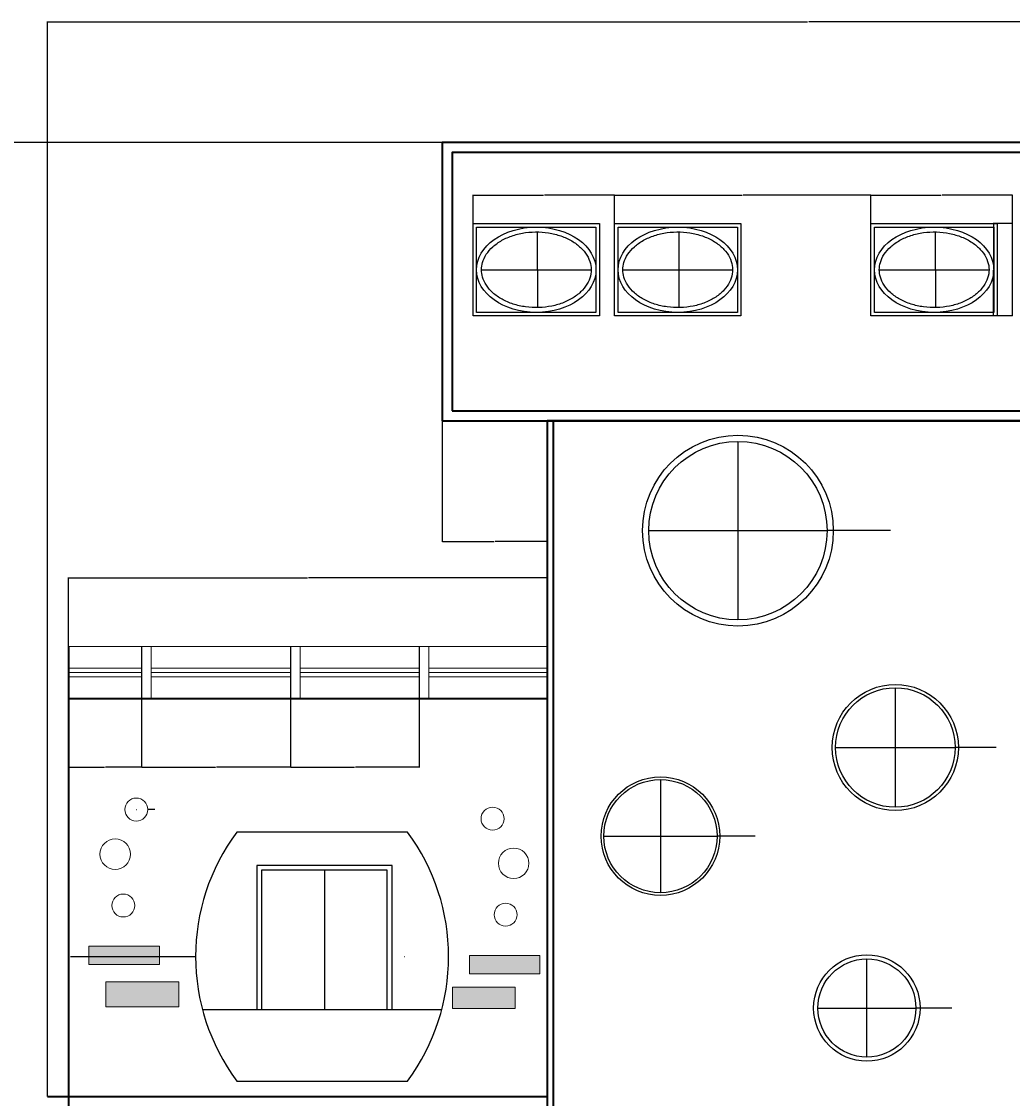
# Model space of a CAD drawing. Units: inches. Extents: x 328 to 2318, y 647 to 2548.
# Tile 4 of 5: x 1040 to 1799, y 1724 to 2548. Entities that reach past the tile are written whole.
import ezdxf

# ---------------------------------------------------------------- set-up
doc = ezdxf.new("R2010")
doc.units = ezdxf.units.IN
doc.header["$MEASUREMENT"] = 0
for name, color, linetype, lineweight in [('A-ANNO-DIMS', 2, 'Continuous', 18), ('A-ELEV', 7, 'Continuous', 35), ('A-ELEV-ORNM', 7, 'Continuous', 18), ('A-GLAZ', 4, 'Continuous', 25), ('A-ROOF', 7, 'Continuous', 35), ('A-ROOF-HRAL', 8, 'Continuous', 18)]:
    doc.layers.add(name, color=color, linetype=linetype, lineweight=lineweight)
doc.layers.add('A-ELEV-ORNM-PATT', color=18, linetype='Continuous', lineweight=13, true_color=0x000000)
doc.styles.get("Standard").update_dxf_attribs({"font": 'arial.ttf'})
doc.dimstyles.get("Standard").update_dxf_attribs({"dimtxt": 0.18, "dimasz": 0.18, "dimexe": 0.18, "dimexo": 0.0625, "dimgap": 0.09, "dimtad": 0, "dimtih": 1, "dimtoh": 1, "dimdec": 4, "dimzin": 0, "dimdsep": 46, "dimtxsty": 'Standard', "dimcen": 0.09, "dimadec": 0, "dimazin": 0, "dimtfac": 1, "dimtdec": 4, "dimtofl": 0, "dimtmove": 0, "dimatfit": 3, "dimfxl": 1, "dimtolj": 1, "dimtzin": 0, "dimarcsym": 0})

# ---------------------------------------------------------------- blocks, each defined once
blk = doc.blocks.new('WIN-ELEV-CURVED-SURROUND')
for p, q in [((162.11, 190.69), (31.57, 190.69)), ((98.64, 161.37), (98.64, 54.8)), ((5.23, 54.8), (188.45, 54.8)), ((31.57, 0), (162.11, 0))]:
    blk.add_line(p, q)
for points in [[(150.48, 54.8), (150.48, 165.07), (46.8, 165.07), (46.8, 54.8)], [(146.78, 54.8), (146.78, 161.37), (50.49, 161.37), (50.49, 54.8)]]:
    blk.add_lwpolyline(points)
for centre, start, end in [((159.76, 95.35), 143.35881, 216.64119), ((33.92, 95.35), 323.35881, 36.64119)]:
    blk.add_arc(centre, 159.76, start, end)
blk = doc.blocks.new('WIN-ELEV-OVAL')
for p, q in [((49.54, 6.37), (49.37, 64.33)), ((6.36, 35.36), (90.36, 35.36))]:
    blk.add_line(p, q)
for points in [[(0, 70.7), (96.72, 70.7), (96.72, 0), (0, 0)], [(2.67, 68.03), (94.06, 68.03), (94.06, 2.67), (2.67, 2.67)]]:
    blk.add_lwpolyline(points, close=True)
blk.add_ellipse((48.36, 35.35), major_axis=(-45.7, 0), ratio=0.715242)
blk.add_open_spline([(6.36, 35.35), (6.36, 33.47), (6.63, 31.58), (7.79, 27.59), (8.77, 25.48), (11.44, 21.43), (13.14, 19.48), (17.17, 15.88), (19.51, 14.22), (24.72, 11.33), (27.59, 10.09), (33.68, 8.11), (36.9, 7.38), (43.51, 6.46), (46.9, 6.28), (53.63, 6.5), (56.98, 6.89), (63.44, 8.21), (66.55, 9.15), (72.35, 11.49), (75.04, 12.9), (79.83, 16.09), (81.94, 17.87), (85.48, 21.67), (86.9, 23.7), (89.04, 27.86), (89.75, 29.99), (90.45, 34.29), (90.45, 36.45), (89.74, 40.75), (89.02, 42.88), (86.88, 47.04), (85.45, 49.06), (81.9, 52.86), (79.79, 54.64), (74.99, 57.83), (72.3, 59.23), (66.49, 61.57), (63.38, 62.5), (56.92, 63.82), (53.57, 64.21), (46.83, 64.41), (43.45, 64.23), (36.84, 63.31), (33.62, 62.57), (27.53, 60.59), (24.67, 59.35), (19.47, 56.45), (17.13, 54.79), (13.1, 51.18), (11.41, 49.23), (8.75, 45.18), (7.78, 43.07), (6.63, 39.09), (6.36, 37.22), (6.36, 35.35)], degree=3, knots=[0, 0, 0, 0, 0.205219, 0.205219, 0.440189, 0.440189, 0.675159, 0.675159, 0.910128, 0.910128, 1.145098, 1.145098, 1.380068, 1.380068, 1.615038, 1.615038, 1.850008, 1.850008, 2.084978, 2.084978, 2.319948, 2.319948, 2.554918, 2.554918, 2.789887, 2.789887, 3.024857, 3.024857, 3.259827, 3.259827, 3.494797, 3.494797, 3.729767, 3.729767, 3.964737, 3.964737, 4.199707, 4.199707, 4.434676, 4.434676, 4.669646, 4.669646, 4.904616, 4.904616, 5.139586, 5.139586, 5.374556, 5.374556, 5.609526, 5.609526, 5.844496, 5.844496, 6.079466, 6.079466, 6.283185, 6.283185, 6.283185, 6.283185])
blk = doc.blocks.new('FACADE-THREE-ROUNDELS')
for centre, radius in [((27.83, 82.27), 8.8), ((11.7, 48.09), 11.7), ((17.88, 8.77), 8.77)]:
    blk.add_circle(centre, radius)
blk = doc.blocks.new('POST-PARAPET')
blk.add_lwpolyline([(0, 0), (7.34, 0), (7.34, 39.76), (0, 39.76)], close=True)
blk = doc.blocks.new('*D8')
at = {"layer": 'A-ANNO-DIMS', "color": 0, "lineweight": -2, "transparency": 16777216}
for p, q in [((1798.98, 2393.44), (1784.36, 2393.44)), ((1784.54, 2393.26), (1784.54, 2358.27)), ((1784.54, 2322.92), (1784.54, 2357.91)), ((1798.98, 2322.74), (1784.36, 2322.74))]:
    blk.add_line(p, q, dxfattribs=at)
at = {"layer": 'A-ANNO-DIMS', "color": 0, "transparency": 16777216}
for points in [[(1784.51, 2393.26), (1784.57, 2393.26), (1784.54, 2393.44)], [(1784.51, 2322.92), (1784.57, 2322.92), (1784.54, 2322.74)]]:
    blk.add_solid(points, dxfattribs=at)
at = {"layer": 'Defpoints', "color": 0, "transparency": 16777216}
for p in [(1784.54, 2393.44), (1799.05, 2393.44), (1799.05, 2322.74)]:
    blk.add_point(p, dxfattribs=at)
at = {"layer": 'A-ANNO-DIMS', "color": 0, "transparency": 16777216, "insert": (1784.54, 2358.09), "char_height": 0.18, "attachment_point": 5}
blk.add_mtext('\\A1;71 TYP.', dxfattribs=at)
blk = doc.blocks.new('*D39')
at = {"layer": 'A-ANNO-DIMS', "color": 0, "lineweight": -2, "transparency": 16777216}
for p, q in [((1060.28, 1725.1), (1060.28, 2548.17)), ((2224.98, 2069.65), (2224.98, 2548.17)), ((1060.46, 2547.99), (1642.17, 2547.99)), ((2224.8, 2547.99), (1643.08, 2547.99))]:
    blk.add_line(p, q, dxfattribs=at)
at = {"layer": 'A-ANNO-DIMS', "color": 0, "transparency": 16777216}
for points in [[(1060.46, 2548.02), (1060.46, 2547.96), (1060.28, 2547.99)], [(2224.8, 2548.02), (2224.8, 2547.96), (2224.98, 2547.99)]]:
    blk.add_solid(points, dxfattribs=at)
at = {"layer": 'Defpoints', "color": 0, "transparency": 16777216}
for p in [(2224.98, 2547.99), (2224.98, 2069.59), (1060.28, 1725.04)]:
    blk.add_point(p, dxfattribs=at)
at = {"layer": 'A-ANNO-DIMS', "color": 0, "transparency": 16777216, "insert": (1642.63, 2547.99), "char_height": 0.18, "attachment_point": 5}
blk.add_mtext('\\A1;1164.7', dxfattribs=at)
blk = doc.blocks.new('*D40')
at = {"layer": 'A-ANNO-DIMS', "color": 0, "lineweight": -2, "transparency": 16777216}
for p, q in [((1362.32, 2455.54), (967.65, 2455.54)), ((967.83, 2455.36), (967.83, 1622.35)), ((967.83, 788.97), (967.83, 1621.98)), ((1076.36, 788.79), (967.65, 788.79))]:
    blk.add_line(p, q, dxfattribs=at)
at = {"layer": 'A-ANNO-DIMS', "color": 0, "transparency": 16777216}
for points in [[(967.8, 2455.36), (967.86, 2455.36), (967.83, 2455.54)], [(967.8, 788.97), (967.86, 788.97), (967.83, 788.79)]]:
    blk.add_solid(points, dxfattribs=at)
at = {"layer": 'Defpoints', "color": 0, "transparency": 16777216}
for p in [(967.83, 2455.54), (1362.39, 2455.54), (1076.43, 788.79)]:
    blk.add_point(p, dxfattribs=at)
at = {"layer": 'A-ANNO-DIMS', "color": 0, "transparency": 16777216, "insert": (967.83, 1622.16), "char_height": 0.18, "attachment_point": 5}
blk.add_mtext('\\A1;1666.7', dxfattribs=at)
blk = doc.blocks.new('*D41')
at = {"layer": 'A-ANNO-DIMS', "color": 0, "lineweight": -2, "transparency": 16777216}
for p, q in [((1076.43, 2029.9), (1076.43, 2122.46)), ((1076.61, 2122.28), (1259.22, 2122.28)), ((1442.63, 2122.28), (1260.01, 2122.28)), ((1442.81, 2029.9), (1442.81, 2122.46))]:
    blk.add_line(p, q, dxfattribs=at)
at = {"layer": 'A-ANNO-DIMS', "color": 0, "transparency": 16777216}
for points in [[(1076.61, 2122.31), (1076.61, 2122.25), (1076.43, 2122.28)], [(1442.63, 2122.31), (1442.63, 2122.25), (1442.81, 2122.28)]]:
    blk.add_solid(points, dxfattribs=at)
at = {"layer": 'Defpoints', "color": 0, "transparency": 16777216}
for p in [(1442.81, 2122.28), (1076.43, 2029.83), (1442.81, 2029.83)]:
    blk.add_point(p, dxfattribs=at)
at = {"layer": 'A-ANNO-DIMS', "color": 0, "transparency": 16777216, "insert": (1259.62, 2122.28), "char_height": 0.18, "attachment_point": 5}
blk.add_mtext('\\A1;366.4', dxfattribs=at)
blk = doc.blocks.new('*D47')
at = {"layer": 'A-ANNO-DIMS', "color": 0, "lineweight": -2, "transparency": 16777216}
for p, q in [((1362.39, 2242.37), (1362.39, 2149.8)), ((1442.81, 2242.37), (1442.81, 2149.8)), ((1362.57, 2149.98), (1402.2, 2149.98)), ((1442.63, 2149.98), (1402.99, 2149.98))]:
    blk.add_line(p, q, dxfattribs=at)
at = {"layer": 'A-ANNO-DIMS', "color": 0, "transparency": 16777216}
for points in [[(1362.57, 2150.01), (1362.57, 2149.95), (1362.39, 2149.98)], [(1442.63, 2150.01), (1442.63, 2149.95), (1442.81, 2149.98)]]:
    blk.add_solid(points, dxfattribs=at)
at = {"layer": 'Defpoints', "color": 0, "transparency": 16777216}
for p in [(1362.39, 2242.43), (1442.81, 2242.43), (1362.39, 2149.98)]:
    blk.add_point(p, dxfattribs=at)
at = {"layer": 'A-ANNO-DIMS', "color": 0, "transparency": 16777216, "insert": (1402.6, 2149.98), "char_height": 0.18, "attachment_point": 5}
blk.add_mtext('\\A1;80.42', dxfattribs=at)
blk = doc.blocks.new('*D50')
at = {"layer": 'A-ANNO-DIMS', "color": 0, "lineweight": -2, "transparency": 16777216}
for p, q in [((1386.14, 2322.8), (1386.14, 2415.37)), ((1386.32, 2415.19), (1439.9, 2415.19)), ((1494.26, 2415.19), (1440.67, 2415.19)), ((1494.44, 2322.8), (1494.44, 2415.37))]:
    blk.add_line(p, q, dxfattribs=at)
at = {"layer": 'A-ANNO-DIMS', "color": 0, "transparency": 16777216}
for points in [[(1386.32, 2415.22), (1386.32, 2415.16), (1386.14, 2415.19)], [(1494.26, 2415.22), (1494.26, 2415.16), (1494.44, 2415.19)]]:
    blk.add_solid(points, dxfattribs=at)
at = {"layer": 'Defpoints', "color": 0, "transparency": 16777216}
for p in [(1494.44, 2415.19), (1386.14, 2322.74), (1494.44, 2322.74)]:
    blk.add_point(p, dxfattribs=at)
at = {"layer": 'A-ANNO-DIMS', "color": 0, "transparency": 16777216, "insert": (1440.29, 2415.19), "char_height": 0.18, "attachment_point": 5}
blk.add_mtext('\\A1;108.3', dxfattribs=at)
blk = doc.blocks.new('*D51')
at = {"layer": 'A-ANNO-DIMS', "color": 0, "lineweight": -2, "transparency": 16777216}
for p, q in [((1494.44, 2322.8), (1494.44, 2415.37)), ((1494.62, 2415.19), (1592.21, 2415.19)), ((1690.56, 2415.19), (1592.98, 2415.19)), ((1690.74, 2322.8), (1690.74, 2415.37))]:
    blk.add_line(p, q, dxfattribs=at)
at = {"layer": 'A-ANNO-DIMS', "color": 0, "transparency": 16777216}
for points in [[(1494.62, 2415.22), (1494.62, 2415.16), (1494.44, 2415.19)], [(1690.56, 2415.22), (1690.56, 2415.16), (1690.74, 2415.19)]]:
    blk.add_solid(points, dxfattribs=at)
at = {"layer": 'Defpoints', "color": 0, "transparency": 16777216}
for p in [(1690.74, 2415.19), (1494.44, 2322.74), (1690.74, 2322.74)]:
    blk.add_point(p, dxfattribs=at)
at = {"layer": 'A-ANNO-DIMS', "color": 0, "transparency": 16777216, "insert": (1592.59, 2415.19), "char_height": 0.18, "attachment_point": 5}
blk.add_mtext('\\A1;196.3', dxfattribs=at)
blk = doc.blocks.new('*D52')
at = {"layer": 'A-ANNO-DIMS', "color": 0, "lineweight": -2, "transparency": 16777216}
for p, q in [((1690.74, 2322.8), (1690.74, 2415.37)), ((1690.92, 2415.19), (1744.51, 2415.19)), ((1798.87, 2415.19), (1745.28, 2415.19)), ((1799.05, 2322.8), (1799.05, 2415.37))]:
    blk.add_line(p, q, dxfattribs=at)
at = {"layer": 'A-ANNO-DIMS', "color": 0, "transparency": 16777216}
for points in [[(1690.92, 2415.22), (1690.92, 2415.16), (1690.74, 2415.19)], [(1798.87, 2415.22), (1798.87, 2415.16), (1799.05, 2415.19)]]:
    blk.add_solid(points, dxfattribs=at)
at = {"layer": 'Defpoints', "color": 0, "transparency": 16777216}
for p in [(1799.05, 2415.19), (1690.74, 2322.74), (1799.05, 2322.74)]:
    blk.add_point(p, dxfattribs=at)
at = {"layer": 'A-ANNO-DIMS', "color": 0, "transparency": 16777216, "insert": (1744.89, 2415.19), "char_height": 0.18, "attachment_point": 5}
blk.add_mtext('\\A1;108.3', dxfattribs=at)
blk = doc.blocks.new('*D62')
at = {"layer": 'A-ANNO-DIMS', "color": 0, "lineweight": -2, "transparency": 16777216}
for p, q in [((1076.43, 2069.53), (1076.43, 1976.96)), ((1132.18, 2069.53), (1132.18, 1976.96)), ((1076.61, 1977.14), (1103.91, 1977.14)), ((1132, 1977.14), (1104.7, 1977.14))]:
    blk.add_line(p, q, dxfattribs=at)
at = {"layer": 'A-ANNO-DIMS', "color": 0, "transparency": 16777216}
for points in [[(1076.61, 1977.17), (1076.61, 1977.11), (1076.43, 1977.14)], [(1132, 1977.17), (1132, 1977.11), (1132.18, 1977.14)]]:
    blk.add_solid(points, dxfattribs=at)
at = {"layer": 'Defpoints', "color": 0, "transparency": 16777216}
for p in [(1076.43, 2069.59), (1132.18, 2069.59), (1076.43, 1977.14)]:
    blk.add_point(p, dxfattribs=at)
at = {"layer": 'A-ANNO-DIMS', "color": 0, "transparency": 16777216, "insert": (1104.3, 1977.14), "char_height": 0.18, "attachment_point": 5}
blk.add_mtext('\\A1;55.76', dxfattribs=at)
blk = doc.blocks.new('*D63')
at = {"layer": 'A-ANNO-DIMS', "color": 0, "lineweight": -2, "transparency": 16777216}
for p, q in [((1132.18, 2069.53), (1132.18, 1976.96)), ((1246.42, 2069.53), (1246.42, 1976.96)), ((1132.36, 1977.14), (1188.85, 1977.14)), ((1246.24, 1977.14), (1189.76, 1977.14))]:
    blk.add_line(p, q, dxfattribs=at)
at = {"layer": 'A-ANNO-DIMS', "color": 0, "transparency": 16777216}
for points in [[(1132.36, 1977.17), (1132.36, 1977.11), (1132.18, 1977.14)], [(1246.24, 1977.17), (1246.24, 1977.11), (1246.42, 1977.14)]]:
    blk.add_solid(points, dxfattribs=at)
at = {"layer": 'Defpoints', "color": 0, "transparency": 16777216}
for p in [(1132.18, 2069.59), (1246.42, 2069.59), (1132.18, 1977.14)]:
    blk.add_point(p, dxfattribs=at)
at = {"layer": 'A-ANNO-DIMS', "color": 0, "transparency": 16777216, "insert": (1189.3, 1977.14), "char_height": 0.18, "attachment_point": 5}
blk.add_mtext('\\A1;114.24', dxfattribs=at)
blk = doc.blocks.new('*D64')
at = {"layer": 'A-ANNO-DIMS', "color": 0, "lineweight": -2, "transparency": 16777216}
for p, q in [((1246.42, 2069.53), (1246.42, 1976.96)), ((1344.93, 2069.53), (1344.93, 1976.96)), ((1246.6, 1977.14), (1295.28, 1977.14)), ((1344.75, 1977.14), (1296.07, 1977.14))]:
    blk.add_line(p, q, dxfattribs=at)
at = {"layer": 'A-ANNO-DIMS', "color": 0, "transparency": 16777216}
for points in [[(1246.6, 1977.17), (1246.6, 1977.11), (1246.42, 1977.14)], [(1344.75, 1977.17), (1344.75, 1977.11), (1344.93, 1977.14)]]:
    blk.add_solid(points, dxfattribs=at)
at = {"layer": 'Defpoints', "color": 0, "transparency": 16777216}
for p in [(1246.42, 2069.59), (1344.93, 2069.59), (1246.42, 1977.14)]:
    blk.add_point(p, dxfattribs=at)
at = {"layer": 'A-ANNO-DIMS', "color": 0, "transparency": 16777216, "insert": (1295.68, 1977.14), "char_height": 0.18, "attachment_point": 5}
blk.add_mtext('\\A1;98.52', dxfattribs=at)
blk = doc.blocks.new('*D68')
at = {"layer": 'A-ANNO-DIMS', "color": 0, "lineweight": -2, "transparency": 16777216}
for p, q in [((1077.79, 1832.22), (1173.47, 1832.22)), ((1333.32, 1832.22), (1333.5, 1832.22)), ((1333.41, 1832.13), (1333.41, 1832.31))]:
    blk.add_line(p, q, dxfattribs=at)
at = {"layer": 'A-ANNO-DIMS', "color": 0, "transparency": 16777216}
blk.add_solid([(1173.47, 1832.25), (1173.47, 1832.19), (1173.65, 1832.22)], dxfattribs=at)
at = {"layer": 'Defpoints', "color": 0, "transparency": 16777216}
for p in [(1173.65, 1832.22), (1333.41, 1832.22)]:
    blk.add_point(p, dxfattribs=at)
at = {"layer": 'A-ANNO-DIMS', "color": 0, "transparency": 16777216, "insert": (1076.99, 1832.22), "char_height": 0.18, "attachment_point": 5}
blk.add_mtext('\\A1;16X R159.76', dxfattribs=at)
blk = doc.blocks.new('*D70')
at = {"layer": 'A-ANNO-DIMS', "color": 0, "lineweight": -2, "transparency": 16777216}
for p, q in [((1128.14, 1944.79), (1128.32, 1944.79)), ((1128.23, 1944.7), (1128.23, 1944.88)), ((1142.31, 1944.79), (1137.21, 1944.79))]:
    blk.add_line(p, q, dxfattribs=at)
at = {"layer": 'A-ANNO-DIMS', "color": 0, "transparency": 16777216}
blk.add_solid([(1137.21, 1944.82), (1137.21, 1944.76), (1137.03, 1944.79)], dxfattribs=at)
at = {"layer": 'Defpoints', "color": 0, "transparency": 16777216}
for p in [(1119.43, 1944.79), (1137.03, 1944.79)]:
    blk.add_point(p, dxfattribs=at)
at = {"layer": 'A-ANNO-DIMS', "color": 0, "transparency": 16777216, "insert": (1143.12, 1944.79), "char_height": 0.18, "attachment_point": 5}
blk.add_mtext('\\A1;16X ∅17.595', dxfattribs=at)
blk = doc.blocks.new('*D72')
at = {"layer": 'A-ANNO-DIMS', "color": 0, "lineweight": -2, "transparency": 16777216}
for p, q in [((1588.76, 2158.33), (1588.94, 2158.33)), ((1588.85, 2158.24), (1588.85, 2158.42)), ((1705.7, 2158.33), (1662.06, 2158.33))]:
    blk.add_line(p, q, dxfattribs=at)
at = {"layer": 'A-ANNO-DIMS', "color": 0, "transparency": 16777216}
blk.add_solid([(1662.06, 2158.36), (1662.06, 2158.3), (1661.88, 2158.33)], dxfattribs=at)
at = {"layer": 'Defpoints', "color": 0, "transparency": 16777216}
for p in [(1515.83, 2158.33), (1661.88, 2158.33)]:
    blk.add_point(p, dxfattribs=at)
at = {"layer": 'A-ANNO-DIMS', "color": 0, "transparency": 16777216, "insert": (1706.26, 2158.33), "char_height": 0.18, "attachment_point": 5}
blk.add_mtext('\\A1;∅146.05', dxfattribs=at)
blk = doc.blocks.new('*D73')
at = {"layer": 'A-ANNO-DIMS', "color": 0, "lineweight": -2, "transparency": 16777216}
for p, q in [((1588.76, 2158.33), (1588.94, 2158.33)), ((1588.85, 2158.24), (1588.85, 2158.42)), ((1698.11, 2158.33), (1657.32, 2158.33))]:
    blk.add_line(p, q, dxfattribs=at)
at = {"layer": 'A-ANNO-DIMS', "color": 0, "transparency": 16777216}
blk.add_solid([(1657.32, 2158.36), (1657.32, 2158.3), (1657.14, 2158.33)], dxfattribs=at)
at = {"layer": 'Defpoints', "color": 0, "transparency": 16777216}
for p in [(1520.57, 2158.33), (1657.14, 2158.33)]:
    blk.add_point(p, dxfattribs=at)
at = {"layer": 'A-ANNO-DIMS', "color": 0, "transparency": 16777216, "insert": (1698.67, 2158.33), "char_height": 0.18, "attachment_point": 5}
blk.add_mtext('\\A1;∅136.57', dxfattribs=at)
blk = doc.blocks.new('*D78')
at = {"layer": 'A-ANNO-DIMS', "color": 0, "lineweight": -2, "transparency": 16777216}
for p, q in [((1709.27, 1992.31), (1709.45, 1992.31)), ((1709.36, 1992.22), (1709.36, 1992.4)), ((1786.65, 1992.31), (1757.84, 1992.31))]:
    blk.add_line(p, q, dxfattribs=at)
at = {"layer": 'A-ANNO-DIMS', "color": 0, "transparency": 16777216}
blk.add_solid([(1757.84, 1992.34), (1757.84, 1992.28), (1757.66, 1992.31)], dxfattribs=at)
at = {"layer": 'Defpoints', "color": 0, "transparency": 16777216}
for p in [(1661.05, 1992.31), (1757.66, 1992.31)]:
    blk.add_point(p, dxfattribs=at)
at = {"layer": 'A-ANNO-DIMS', "color": 0, "transparency": 16777216, "insert": (1787.12, 1992.31), "char_height": 0.18, "attachment_point": 5}
blk.add_mtext('\\A1;∅96.61', dxfattribs=at)
blk = doc.blocks.new('*D79')
at = {"layer": 'A-ANNO-DIMS', "color": 0, "lineweight": -2, "transparency": 16777216}
for p, q in [((1709.27, 1992.31), (1709.45, 1992.31)), ((1709.36, 1992.22), (1709.36, 1992.4)), ((1782.57, 1992.31), (1755.29, 1992.31))]:
    blk.add_line(p, q, dxfattribs=at)
at = {"layer": 'A-ANNO-DIMS', "color": 0, "transparency": 16777216}
blk.add_solid([(1755.29, 1992.34), (1755.29, 1992.28), (1755.11, 1992.31)], dxfattribs=at)
at = {"layer": 'Defpoints', "color": 0, "transparency": 16777216}
for p in [(1663.6, 1992.31), (1755.11, 1992.31)]:
    blk.add_point(p, dxfattribs=at)
at = {"layer": 'A-ANNO-DIMS', "color": 0, "transparency": 16777216, "insert": (1783.04, 1992.31), "char_height": 0.18, "attachment_point": 5}
blk.add_mtext('\\A1;∅91.51', dxfattribs=at)
blk = doc.blocks.new('*D80')
at = {"layer": 'A-ANNO-DIMS', "color": 0, "lineweight": -2, "transparency": 16777216}
for p, q in [((1529.44, 1924.41), (1529.62, 1924.41)), ((1529.53, 1924.32), (1529.53, 1924.5)), ((1602.18, 1924.41), (1575.12, 1924.41))]:
    blk.add_line(p, q, dxfattribs=at)
at = {"layer": 'A-ANNO-DIMS', "color": 0, "transparency": 16777216}
blk.add_solid([(1575.12, 1924.44), (1575.12, 1924.38), (1574.94, 1924.41)], dxfattribs=at)
at = {"layer": 'Defpoints', "color": 0, "transparency": 16777216}
for p in [(1484.13, 1924.41), (1574.94, 1924.41)]:
    blk.add_point(p, dxfattribs=at)
at = {"layer": 'A-ANNO-DIMS', "color": 0, "transparency": 16777216, "insert": (1602.6, 1924.41), "char_height": 0.18, "attachment_point": 5}
blk.add_mtext('\\A1;∅90.8', dxfattribs=at)
blk = doc.blocks.new('*D81')
at = {"layer": 'A-ANNO-DIMS', "color": 0, "lineweight": -2, "transparency": 16777216}
for p, q in [((1529.44, 1924.41), (1529.62, 1924.41)), ((1529.53, 1924.32), (1529.53, 1924.5)), ((1598.88, 1924.41), (1573.05, 1924.41))]:
    blk.add_line(p, q, dxfattribs=at)
at = {"layer": 'A-ANNO-DIMS', "color": 0, "transparency": 16777216}
blk.add_solid([(1573.05, 1924.44), (1573.05, 1924.38), (1572.87, 1924.41)], dxfattribs=at)
at = {"layer": 'Defpoints', "color": 0, "transparency": 16777216}
for p in [(1486.19, 1924.41), (1572.87, 1924.41)]:
    blk.add_point(p, dxfattribs=at)
at = {"layer": 'A-ANNO-DIMS', "color": 0, "transparency": 16777216, "insert": (1599.37, 1924.41), "char_height": 0.18, "attachment_point": 5}
blk.add_mtext('\\A1;∅86.68', dxfattribs=at)
blk = doc.blocks.new('*D82')
at = {"layer": 'A-ANNO-DIMS', "color": 0, "lineweight": -2, "transparency": 16777216}
for p, q in [((1687.48, 1792.81), (1687.66, 1792.81)), ((1687.57, 1792.72), (1687.57, 1792.9)), ((1752.75, 1792.81), (1728.49, 1792.81))]:
    blk.add_line(p, q, dxfattribs=at)
at = {"layer": 'A-ANNO-DIMS', "color": 0, "transparency": 16777216}
blk.add_solid([(1728.49, 1792.84), (1728.49, 1792.78), (1728.31, 1792.81)], dxfattribs=at)
at = {"layer": 'Defpoints', "color": 0, "transparency": 16777216}
for p in [(1646.84, 1792.81), (1728.31, 1792.81)]:
    blk.add_point(p, dxfattribs=at)
at = {"layer": 'A-ANNO-DIMS', "color": 0, "transparency": 16777216, "insert": (1753.25, 1792.81), "char_height": 0.18, "attachment_point": 5}
blk.add_mtext('\\A1;∅81.48', dxfattribs=at)
blk = doc.blocks.new('*D83')
at = {"layer": 'A-ANNO-DIMS', "color": 0, "lineweight": -2, "transparency": 16777216}
for p, q in [((1687.48, 1792.81), (1687.66, 1792.81)), ((1687.57, 1792.72), (1687.57, 1792.9)), ((1747.66, 1792.81), (1725.31, 1792.81))]:
    blk.add_line(p, q, dxfattribs=at)
at = {"layer": 'A-ANNO-DIMS', "color": 0, "transparency": 16777216}
blk.add_solid([(1725.31, 1792.84), (1725.31, 1792.78), (1725.13, 1792.81)], dxfattribs=at)
at = {"layer": 'Defpoints', "color": 0, "transparency": 16777216}
for p in [(1650.02, 1792.81), (1725.13, 1792.81)]:
    blk.add_point(p, dxfattribs=at)
at = {"layer": 'A-ANNO-DIMS', "color": 0, "transparency": 16777216, "insert": (1748.06, 1792.81), "char_height": 0.18, "attachment_point": 5}
blk.add_mtext('\\A1;∅75.1', dxfattribs=at)

msp = doc.modelspace()

# ---------------------------------------------------------------- hatches: boundary and pattern name
at = {"layer": 'A-ELEV-ORNM-PATT'}
h = msp.add_hatch(color=256, dxfattribs=at)
h.dxf.hatch_style = 1
h.paths.add_polyline_path([(1160.8736, 1194.017), (1104.946, 1194.017), (1104.946, 1174.8467), (1160.8736, 1174.8467)])
h.paths.add_polyline_path([(1145.9162, 1221.3103), (1091.9395, 1221.3103), (1091.9395, 1207.3388), (1145.9162, 1207.3388)])
h.paths.add_polyline_path([(1418.337, 1190.1501), (1370.4156, 1190.1501), (1370.4156, 1173.7241), (1418.337, 1173.7241)])
h.paths.add_polyline_path([(1437.3105, 1214.299), (1383.3339, 1214.299), (1383.3339, 1200.3274), (1437.3105, 1200.3274)])
h.paths.add_polyline_path([(1418.337, 1499.5227), (1370.4156, 1499.5227), (1370.4156, 1483.0967), (1418.337, 1483.0967)])
h.paths.add_polyline_path([(1437.3105, 1523.6716), (1383.3339, 1523.6716), (1383.3339, 1509.7), (1437.3105, 1509.7)])
h.paths.add_polyline_path([(1145.9162, 1530.683), (1091.9395, 1530.683), (1091.9395, 1516.7114), (1145.9162, 1516.7114)])
h.paths.add_polyline_path([(1160.8736, 1503.3896), (1104.946, 1503.3896), (1104.946, 1484.2194), (1160.8736, 1484.2194)])
h.paths.add_polyline_path([(1160.8736, 1812.7623), (1104.946, 1812.7623), (1104.946, 1793.592), (1160.8736, 1793.592)])
h.paths.add_polyline_path([(1145.9162, 1840.0556), (1091.9395, 1840.0556), (1091.9395, 1826.084), (1145.9162, 1826.084)])
h.paths.add_polyline_path([(1437.3105, 1833.0442), (1383.3339, 1833.0442), (1383.3339, 1819.0726), (1437.3105, 1819.0726)])
h.paths.add_polyline_path([(1418.337, 1808.8953), (1370.4156, 1808.8953), (1370.4156, 1792.4693), (1418.337, 1792.4693)])
h.paths.add_polyline_path([(1145.9162, 908.3867), (1091.9395, 908.3867), (1091.9395, 894.4151), (1145.9162, 894.4151)])
h.paths.add_polyline_path([(1160.8736, 881.0933), (1104.946, 881.0933), (1104.946, 861.923), (1160.8736, 861.923)])
h.paths.add_polyline_path([(1418.337, 877.2264), (1370.4156, 877.2264), (1370.4156, 860.8004), (1418.337, 860.8004)])
h.paths.add_polyline_path([(1437.3105, 901.3753), (1383.3339, 901.3753), (1383.3339, 887.4037), (1437.3105, 887.4037)])
h.paths.add_polyline_path([(1926.897, 881.0933), (1870.9694, 881.0933), (1870.9694, 861.923), (1926.897, 861.923)])
h.paths.add_polyline_path([(1911.9396, 908.3867), (1857.9629, 908.3867), (1857.9629, 894.4151), (1911.9396, 894.4151)])
h.paths.add_polyline_path([(2184.3603, 877.2264), (2136.439, 877.2264), (2136.439, 860.8004), (2184.3603, 860.8004)])
h.paths.add_polyline_path([(2203.3339, 901.3753), (2149.3572, 901.3753), (2149.3572, 887.4037), (2203.3339, 887.4037)])
h.paths.add_polyline_path([(2184.3603, 1190.1501), (2136.439, 1190.1501), (2136.439, 1173.7241), (2184.3603, 1173.7241)])
h.paths.add_polyline_path([(2203.3339, 1214.299), (2149.3572, 1214.299), (2149.3572, 1200.3274), (2203.3339, 1200.3274)])
h.paths.add_polyline_path([(1911.9396, 1221.3103), (1857.9629, 1221.3103), (1857.9629, 1207.3388), (1911.9396, 1207.3388)])
h.paths.add_polyline_path([(1926.897, 1194.017), (1870.9694, 1194.017), (1870.9694, 1174.8467), (1926.897, 1174.8467)])
h.paths.add_polyline_path([(1926.897, 1503.3896), (1870.9694, 1503.3896), (1870.9694, 1484.2194), (1926.897, 1484.2194)])
h.paths.add_polyline_path([(1911.9396, 1530.683), (1857.9629, 1530.683), (1857.9629, 1516.7114), (1911.9396, 1516.7114)])
h.paths.add_polyline_path([(2184.3603, 1499.5227), (2136.439, 1499.5227), (2136.439, 1483.0967), (2184.3603, 1483.0967)])
h.paths.add_polyline_path([(2203.3339, 1523.6716), (2149.3572, 1523.6716), (2149.3572, 1509.7), (2203.3339, 1509.7)])
h.paths.add_polyline_path([(1926.897, 1812.7623), (1870.9694, 1812.7623), (1870.9694, 1793.592), (1926.897, 1793.592)])
h.paths.add_polyline_path([(1911.9396, 1840.0556), (1857.9629, 1840.0556), (1857.9629, 1826.084), (1911.9396, 1826.084)])
h.paths.add_polyline_path([(2184.3603, 1808.8953), (2136.439, 1808.8953), (2136.439, 1792.4693), (2184.3603, 1792.4693)])
h.paths.add_polyline_path([(2203.3339, 1833.0442), (2149.3572, 1833.0442), (2149.3572, 1819.0726), (2203.3339, 1819.0726)])

# ---------------------------------------------------------------- linework, layer by layer
at = {"layer": 'A-ELEV'}
for p, q in [((1842.45, 2242.4288), (1442.8075, 2242.4288)), ((1442.8075, 2242.4288), (1442.8075, 1101.7147)), ((1447.3872, 2242.4288), (1447.3872, 1106.2944)), ((1076.4266, 2069.5914), (1076.4266, 788.791)), ((1076.4266, 2029.8325), (1442.8075, 2029.8325)), ((1060.276, 1725.0396), (1442.8075, 1725.0396))]:
    msp.add_line(p, q, dxfattribs=at)
at = {"layer": 'A-ELEV-ORNM'}
for points in [[(1091.9395, 1840.0556), (1145.9162, 1840.0556), (1145.9162, 1826.084), (1091.9395, 1826.084)], [(1437.3105, 1833.0442), (1383.3339, 1833.0442), (1383.3339, 1819.0726), (1437.3105, 1819.0726)], [(1104.946, 1812.7623), (1160.8736, 1812.7623), (1160.8736, 1793.592), (1104.946, 1793.592)], [(1418.337, 1808.8953), (1370.4156, 1808.8953), (1370.4156, 1792.4693), (1418.337, 1792.4693)]]:
    msp.add_lwpolyline(points, close=True, dxfattribs=at)
at = {"layer": 'A-GLAZ'}
for p, q in [((1588.8547, 2226.6132), (1588.8547, 2090.0471)), ((1520.5717, 2158.3301), (1657.1378, 2158.3301)), ((1709.3563, 2038.0638), (1709.3563, 1946.5499)), ((1663.5993, 1992.3068), (1755.1132, 1992.3068)), ((1529.5327, 1967.7532), (1529.5327, 1881.071)), ((1486.1916, 1924.4121), (1572.8738, 1924.4121)), ((1687.5736, 1755.2567), (1687.5736, 1830.3607)), ((1650.0217, 1792.8087), (1725.1256, 1792.8087))]:
    msp.add_line(p, q, dxfattribs=at)
for centre, radius in [((1588.8547, 2158.3301), 73.0256), ((1588.8547, 2158.3301), 68.2831), ((1709.3563, 1992.3068), 48.3057), ((1709.3563, 1992.3068), 45.7569), ((1529.5327, 1924.4121), 45.403), ((1529.5327, 1924.4121), 43.3411), ((1687.5736, 1792.8087), 40.7377), ((1687.5736, 1792.8087), 37.552)]:
    msp.add_circle(centre, radius, dxfattribs=at)
at = {"layer": 'A-ROOF'}
for points in [[(1362.3871, 2242.4288), (1922.9232, 2242.4288), (1922.9232, 2455.5387), (1362.3871, 2455.5387)], [(1370.0417, 2250.0835), (1915.2686, 2250.0835), (1915.2686, 2447.8841), (1370.0417, 2447.8841)]]:
    msp.add_lwpolyline(points, close=True, dxfattribs=at)
at = {"layer": 'A-ROOF-HRAL'}
for p, q in [((1076.4266, 2069.5914), (1442.8075, 2069.5914)), ((1076.4266, 2053.0614), (1132.1823, 2053.0614)), ((1132.1823, 2049.712), (1076.4266, 2049.712)), ((1076.4266, 2049.712), (1132.1823, 2049.712)), ((1076.4266, 2046.4313), (1132.1823, 2046.4313)), ((1139.5186, 2053.0614), (1246.4185, 2053.0614)), ((1139.5186, 2049.712), (1246.4185, 2049.712)), ((1139.5186, 2046.4313), (1246.4185, 2046.4313)), ((1253.7548, 2053.0614), (1344.9342, 2053.0614)), ((1253.7548, 2049.712), (1344.9342, 2049.712)), ((1253.7548, 2046.4313), (1344.9342, 2046.4313)), ((1352.2704, 2053.0614), (1442.8075, 2053.0614)), ((1352.2704, 2049.712), (1442.8075, 2049.712)), ((1352.2704, 2046.4313), (1442.8075, 2046.4313))]:
    msp.add_line(p, q, dxfattribs=at)

# ---------------------------------------------------------------- block references
at = {"layer": 'A-ELEV-ORNM'}
msp.add_blockref('FACADE-THREE-ROUNDELS', (1100.4017, 1862.5181), dxfattribs=at)
at = {"layer": 'A-ELEV-ORNM', "extrusion": (0, 0, -1), "zscale": -1}
msp.add_blockref('FACADE-THREE-ROUNDELS', (-1428.8484, 1855.5067), dxfattribs=at)
at = {"layer": 'A-GLAZ'}
for name, p in [('WIN-ELEV-OVAL', (1386.1366, 2322.7365)), ('WIN-ELEV-OVAL', (1494.4424, 2322.7365)), ('WIN-ELEV-OVAL', (1690.741, 2322.7365)), ('WIN-ELEV-CURVED-SURROUND', (1173.6493, 1736.8753))]:
    msp.add_blockref(name, p, dxfattribs=at)
at = {"layer": 'A-ROOF-HRAL'}
for p in [(1132.1823, 2029.8325), (1246.4185, 2029.8325), (1344.9342, 2029.8325)]:
    msp.add_blockref('POST-PARAPET', p, dxfattribs=at)

# ---------------------------------------------------------------- dimensions: what is measured, and where the dimension line sits
at = {"layer": 'A-ANNO-DIMS'}
for base, p1, p2, picture, middle in [((2224.9815, 2547.9887), (1060.276, 1725.0396), (2224.9815, 2069.5914), '*D39', (1642.6287, 2547.9887)), ((1494.4424, 2415.1865), (1386.1366, 2322.7365), (1494.4424, 2322.7365), '*D50', (1440.2895, 2415.1865)), ((1690.741, 2415.1865), (1494.4424, 2322.7365), (1690.741, 2322.7365), '*D51', (1592.5917, 2415.1865)), ((1799.0469, 2415.1865), (1690.741, 2322.7365), (1799.0469, 2322.7365), '*D52', (1744.894, 2415.1865)), ((1442.8075, 2122.2825), (1076.4266, 2029.8325), (1442.8075, 2029.8325), '*D41', (1259.6171, 2122.2825))]:
    dim = msp.add_linear_dim(base=base, p1=p1, p2=p2, dimstyle='Standard', override={"dimdec": 1, "dimlfac": 1, "dimrnd": 0, "dimzin": 0, "dimdsep": 46, "dimlunit": 2}, dxfattribs=at)
    dim.commit()
    dim.dimension.update_dxf_attribs({"geometry": picture, "text_midpoint": middle})
for base, p1, p2, angle, override, picture, middle in [((967.826, 2455.5387), (1076.4266, 788.791), (1362.3871, 2455.5387), 90, {"dimdec": 1, "dimlfac": 1, "dimrnd": 0, "dimzin": 0, "dimdsep": 46, "dimlunit": 2}, '*D40', (967.826, 1622.1648)), ((1362.3871, 2149.9788), (1442.8075, 2242.4288), (1362.3871, 2242.4288), 180, {"dimdec": 2, "dimlfac": 1, "dimrnd": 0, "dimzin": 0, "dimdsep": 46, "dimlunit": 2}, '*D47', (1402.5973, 2149.9788)), ((1076.4266, 1977.1414), (1132.1823, 2069.5914), (1076.4266, 2069.5914), 180, {"dimdec": 2, "dimlfac": 1, "dimrnd": 0, "dimzin": 0, "dimdsep": 46, "dimlunit": 2}, '*D62', (1104.3045, 1977.1414)), ((1132.1823, 1977.1414), (1246.4185, 2069.5914), (1132.1823, 2069.5914), 180, {"dimdec": 2, "dimlfac": 1, "dimrnd": 0, "dimzin": 0, "dimdsep": 46, "dimlunit": 2}, '*D63', (1189.3004, 1977.1414)), ((1246.4185, 1977.1414), (1344.9342, 2069.5914), (1246.4185, 2069.5914), 180, {"dimdec": 2, "dimlfac": 1, "dimrnd": 0, "dimzin": 0, "dimdsep": 46, "dimlunit": 2}, '*D64', (1295.6763, 1977.1414))]:
    dim = msp.add_linear_dim(base=base, p1=p1, p2=p2, angle=angle, dimstyle='Standard', override=override, dxfattribs=at)
    dim.commit()
    dim.dimension.update_dxf_attribs({"geometry": picture, "text_midpoint": middle})
dim = msp.add_linear_dim(base=(1784.5385, 2393.4351), p1=(1799.0469, 2322.7365), p2=(1799.0469, 2393.4351), angle=90, text='<> TYP.', dimstyle='Standard', override={"dimdec": 0, "dimlfac": 1, "dimrnd": 0, "dimzin": 0, "dimdsep": 46, "dimlunit": 2}, dxfattribs=at)
dim.commit()
dim.dimension.update_dxf_attribs({"geometry": '*D8', "text_midpoint": (1784.5385, 2358.0858)})
for p1, p2, override, picture, middle in [((1515.8291, 2158.3302), (1661.8803, 2158.33), {"dimdec": 2, "dimlfac": 1, "dimrnd": 0, "dimzin": 0, "dimdsep": 46, "dimlunit": 2}, '*D72', (1705.6957, 2158.3299)), ((1520.5717, 2158.3302), (1657.1378, 2158.33), {"dimdec": 2, "dimlfac": 1, "dimrnd": 0, "dimzin": 0, "dimdsep": 46, "dimlunit": 2}, '*D73', (1698.1076, 2158.3299)), ((1661.0506, 1992.3066), (1757.6619, 1992.307), {"dimdec": 2, "dimlfac": 1, "dimrnd": 0, "dimzin": 0, "dimdsep": 46, "dimlunit": 2}, '*D78', (1786.6453, 1992.3071)), ((1663.5993, 1992.3066), (1755.1132, 1992.307), {"dimdec": 2, "dimlfac": 1, "dimrnd": 0, "dimzin": 0, "dimdsep": 46, "dimlunit": 2}, '*D79', (1782.5674, 1992.3071)), ((1484.1297, 1924.4122), (1574.9357, 1924.412), {"dimdec": 1, "dimlfac": 1, "dimrnd": 0, "dimzin": 0, "dimdsep": 46, "dimlunit": 2}, '*D80', (1602.1775, 1924.412)), ((1486.1916, 1924.4122), (1572.8738, 1924.412), {"dimdec": 2, "dimlfac": 1, "dimrnd": 0, "dimzin": 0, "dimdsep": 46, "dimlunit": 2}, '*D81', (1598.8785, 1924.412)), ((1646.8359, 1792.8084), (1728.3114, 1792.809), {"dimdec": 2, "dimlfac": 1, "dimrnd": 0, "dimzin": 0, "dimdsep": 46, "dimlunit": 2}, '*D82', (1752.754, 1792.8092)), ((1650.0217, 1792.8084), (1725.1256, 1792.809), {"dimdec": 1, "dimlfac": 1, "dimrnd": 0, "dimzin": 0, "dimdsep": 46, "dimlunit": 2}, '*D83', (1747.6568, 1792.8092))]:
    dim = msp.add_diameter_dim_2p(p1=p1, p2=p2, dimstyle='Standard', override=override, dxfattribs=at)
    dim.commit()
    dim.dimension.update_dxf_attribs({"geometry": picture, "text_midpoint": middle, "dimtype": 163})
dim = msp.add_diameter_dim_2p(p1=(1119.4341, 1944.7904), p2=(1137.0291, 1944.79), text='16X <>', dimstyle='Standard', override={"dimdec": 3, "dimlfac": 1, "dimrnd": 0, "dimzin": 0, "dimdsep": 46, "dimlunit": 2}, dxfattribs=at)
dim.commit()
dim.dimension.update_dxf_attribs({"geometry": '*D70', "text_midpoint": (1142.3076, 1944.7899), "dimtype": 163})
dim = msp.add_radius_dim(center=(1333.4097, 1832.2206), mpoint=(1173.6493, 1832.221), text='16X <>', dimstyle='Standard', override={"dimdec": 2, "dimlfac": 1, "dimrnd": 0, "dimzin": 0, "dimdsep": 46, "dimlunit": 2}, dxfattribs=at)
dim.commit()
dim.dimension.update_dxf_attribs({"geometry": '*D68', "text_midpoint": (1077.7931, 1832.2213), "dimtype": 164})

doc.saveas('drawing.dxf')
